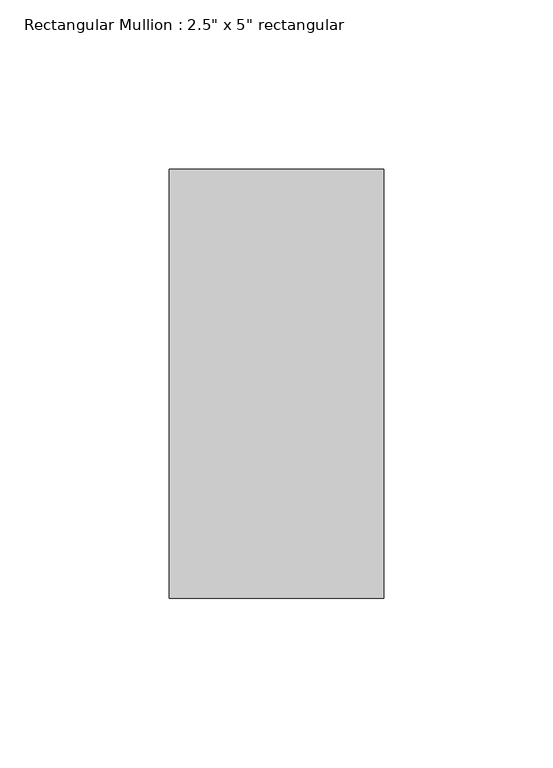
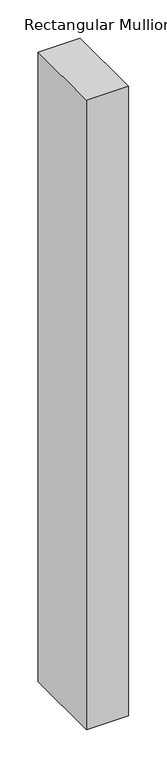
"""IFC4 building model written with IfcOpenShell, lengths in millimetres: member geometry."""

from ifc_helpers import new_model, si_unit, frame, origin, place, context, project, spatial, polyline, outline, extrude, source, transform, mapped, element, save


def member_2251cb41(model_context):
    return source(origin(), model_context, "Body", "SweptSolid", [
        extrude(outline(polyline([(31.75, 63.5), (31.75, -63.5), (-31.75, -63.5), (-31.75, 63.5), (31.75, 63.5)])), frame((0.0, 0.0, -1004.616916), z_axis=(0.0, 0.0, 1.0), x_axis=(1.0, 0.0, 0.0)), (0.0, 0.0, 1.0), 1004.616916),
    ])


if __name__ == "__main__":
    model = new_model("IFC4")
    model_context = context("Model", 3, world=origin())
    ifc_project = project(units=[si_unit("LENGTHUNIT", "METRE", prefix="MILLI")], contexts=[model_context])
    site = spatial("IfcSite", under=ifc_project)
    building = spatial("IfcBuilding", under=site)
    placement = place(None, origin())
    member_shape = member_2251cb41(model_context)
    element("IfcMember", 1, ObjectType="Rectangular Mullion : 2.5\" x 5\" rectangular", at=placement, inside=building, context=model_context, shape_type="MappedRepresentation", body=[
        mapped(member_shape, transform((0.0, 0.0, 0.0), x_axis=(1.0, 0.0, 0.0), y_axis=(0.0, 1.0, 0.0), z_axis=(0.0, 0.0, 1.0))),
    ])
    save(model, "model.ifc")

# Revit data of these elements
# Type "Rectangular Mullion : 2.5\" x 5\" rectangular"
#   built-in parameter 1007304 = 0.416667 (stored number, unit not read)
#   built-in parameter 1007301 = 0.104167 (stored number, unit not read)
#   built-in parameter 1007300 = 0.104167 (stored number, unit not read)
# Element 1 (IfcMember, "Rectangular Mullion : 2.5\" x 5\" rectangular")
#   Materials on its faces: "Aluminum"
# Materials
#   "Aluminum": class "Metal", colour RGB 247 247 247, transparency 0, Description = "Aluminum 6061", Cost = 0
